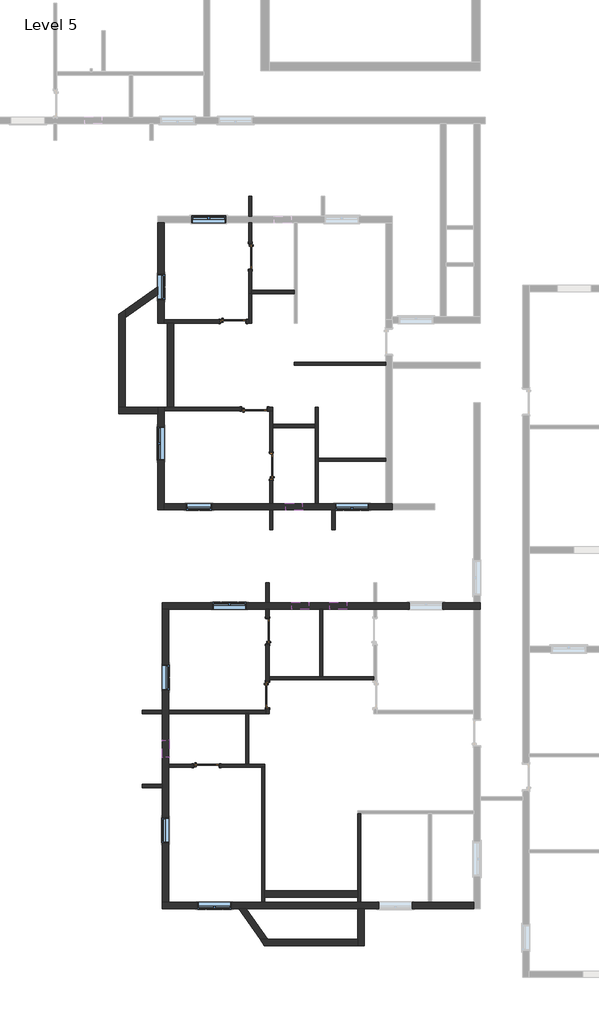
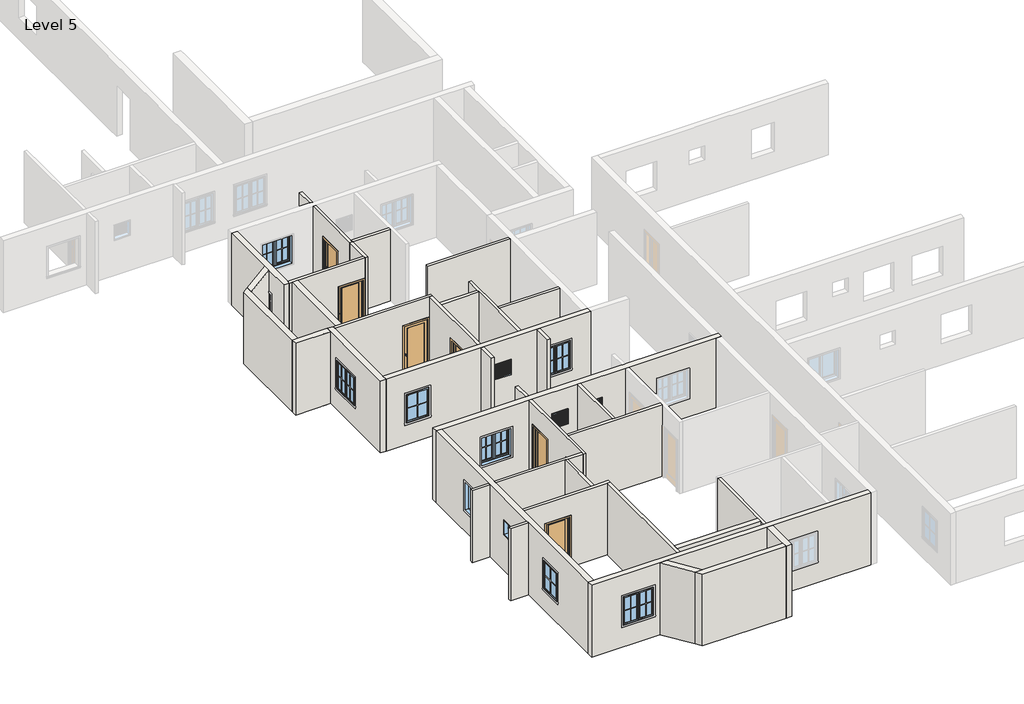
# One storey, part 1 of 7: 39 walls, 13 windows, 7 doors.
"""IFC4 building model written with IfcOpenShell, lengths in millimetres."""

from ifc_helpers import new_model, si_unit, frame, origin, place, context, project, spatial, polyline, outline, extrude, faceted_brep, transform, mapped, element, save
from components import door_3c6ab76a, door_a3feeac7, window_272f20d6, window_casement_double_4_x_4_af3140d2, window_f2d8fef0

model = new_model("IFC4")

# Units and contexts
model_context = context("Model", 3, world=origin())
ifc_project = project(units=[si_unit("LENGTHUNIT", "METRE", prefix="MILLI")], contexts=[model_context])

# Site, building, storey
site = spatial("IfcSite", under=ifc_project)
building = spatial("IfcBuilding", under=site)
storey = spatial("IfcBuildingStorey", under=building, Name="Level 5", Elevation=6400.8)

# Doors
placement = place(None, origin())
door_shape = door_3c6ab76a(model_context)
element("IfcDoor", 1, ObjectType="Door-Interior-Single-1_Panel-Wood : 2'6\" x 7' door", at=placement, inside=storey, context=model_context, shape_type="MappedRepresentation", body=[
    mapped(door_shape, transform((-4216.6759469, -3460.4538828, 6400.8), x_axis=(0.0, -1.0, 0.0), y_axis=(1.0, 0.0, 0.0), z_axis=(0.0, 0.0, 1.0))),
])
element("IfcDoor", 2, ObjectType="Door-Interior-Single-1_Panel-Wood : 2'6\" x 7' door", at=placement, inside=storey, context=model_context, shape_type="MappedRepresentation", body=[
    mapped(door_shape, transform((-5797.8259469, -21840.5288828, 6400.8), x_axis=(1.0, 0.0, 0.0), y_axis=(0.0, 1.0, 0.0), z_axis=(0.0, 0.0, 1.0))),
])
door_2_shape = door_a3feeac7(model_context)
element("IfcDoor", 3, ObjectType="Door-Interior-Single-1_Panel-Wood : 2'6\" x 7' door", at=placement, inside=storey, context=model_context, shape_type="MappedRepresentation", body=[
    mapped(door_2_shape, transform((-3454.6759469, -11032.8288828, 6400.8), x_axis=(0.0, 1.0, 0.0), y_axis=(-1.0, 0.0, 0.0), z_axis=(0.0, 0.0, 1.0))),
])
element("IfcDoor", 4, ObjectType="Door-Interior-Single-1_Panel-Wood : 2'6\" x 7' door", at=placement, inside=storey, context=model_context, shape_type="MappedRepresentation", body=[
    mapped(door_2_shape, transform((-3594.3759469, -16985.9538828, 6400.8), x_axis=(0.0, 1.0, 0.0), y_axis=(-1.0, 0.0, 0.0), z_axis=(0.0, 0.0, 1.0))),
])
element("IfcDoor", 5, ObjectType="Door-Interior-Single-1_Panel-Wood : 36\" x 84\"", at=placement, inside=storey, context=model_context, shape_type="MappedRepresentation", body=[
    mapped(door_shape, transform((-4829.4509469, -5800.4288828, 6400.8), x_axis=(1.0, 0.0, 0.0), y_axis=(0.0, 1.0, 0.0), z_axis=(0.0, 0.0, 1.0))),
])
element("IfcDoor", 6, ObjectType="Door-Interior-Single-1_Panel-Wood : 36\" x 84\"", at=placement, inside=storey, context=model_context, shape_type="MappedRepresentation", body=[
    mapped(door_2_shape, transform((-4067.4509469, -8969.0788828, 6400.8), x_axis=(1.0, 0.0, 0.0), y_axis=(0.0, 1.0, 0.0), z_axis=(0.0, 0.0, 1.0))),
])
element("IfcDoor", 7, ObjectType="Door-Interior-Single-1_Panel-Wood : 36\" x 84\"", at=placement, inside=storey, context=model_context, shape_type="MappedRepresentation", body=[
    mapped(door_2_shape, transform((-3600.7259469, -19291.0038828, 6400.8), x_axis=(0.0, -1.0, 0.0), y_axis=(1.0, 0.0, 0.0), z_axis=(0.0, 0.0, 1.0))),
])

# Walls
element("IfcWall", 8, ObjectType="4.5\" wall", at=placement, inside=storey, context=model_context, shape_type="Brep", body=[
    faceted_brep([(-4277.0009469, -4793.9538828, 9448.8), (-4277.0009469, -2241.2538828, 9448.8), (-4277.0009469, -2241.2538828, 6400.8), (-4277.0009469, -2977.8538828, 6400.8), (-4277.0009469, -2977.8538828, 8559.8), (-4277.0009469, -3943.0538828, 8559.8), (-4277.0009469, -3943.0538828, 6400.8), (-4277.0009469, -4793.9538828, 6400.8), (-4162.7009469, -2241.2538828, 9448.8), (-4162.7009469, -4679.6538828, 9448.8), (-4162.7009469, -4793.9538828, 9448.8), (-4162.7009469, -4793.9538828, 6400.8), (-4162.7009469, -4679.6538828, 6400.8), (-4162.7009469, -3943.0538828, 6400.8), (-4162.7009469, -3943.0538828, 8559.8), (-4162.7009469, -2977.8538828, 8559.8), (-4162.7009469, -2977.8538828, 6400.8), (-4162.7009469, -2241.2538828, 6400.8)], [[[0, 1, 2, 3, 4, 5, 6, 7]], [[8, 9, 10, 11, 12, 13, 14, 15, 16, 17]], [[2, 17, 16, 3]], [[11, 7, 6, 13, 12]], [[1, 0, 10, 9, 8]], [[2, 1, 8, 17]], [[0, 7, 11, 10]], [[5, 14, 13, 6]], [[14, 5, 4, 15]], [[15, 4, 3, 16]]]),
])
element("IfcWall", 9, ObjectType="4.5\" wall", at=placement, inside=storey, context=model_context, shape_type="Brep", body=[
    faceted_brep([(-4277.0009469, -4793.9538828, 6400.8), (-4277.0009469, -5746.4538828, 6400.8), (-4277.0009469, -5860.7538828, 6400.8), (-4277.0009469, -5860.7538828, 9448.8), (-4277.0009469, -5746.4538828, 9448.8), (-4277.0009469, -4793.9538828, 9448.8), (-4162.7009469, -4793.9538828, 6400.8), (-4162.7009469, -4793.9538828, 9448.8), (-4162.7009469, -5860.7538828, 9448.8), (-4162.7009469, -5860.7538828, 6400.8)], [[[0, 1, 2, 3, 4, 5]], [[6, 7, 8, 9]], [[2, 1, 0, 6, 9]], [[5, 4, 3, 8, 7]], [[0, 5, 7, 6]], [[3, 2, 9, 8]]]),
])
element("IfcWall", 10, ObjectType="4.5\" wall", at=placement, inside=storey, context=model_context, shape_type="Brep", body=[
    faceted_brep([(-7325.0009469, -5746.4538828, 9448.8), (-4277.0009469, -5746.4538828, 9448.8), (-4277.0009469, -5746.4538828, 6400.8), (-4346.8509469, -5746.4538828, 6400.8), (-4346.8509469, -5746.4538828, 8559.8), (-5312.0509469, -5746.4538828, 8559.8), (-5312.0509469, -5746.4538828, 6400.8), (-7325.0009469, -5746.4538828, 6400.8), (-4277.0009469, -5860.7538828, 9448.8), (-6982.1009469, -5860.7538828, 9448.8), (-7210.7009469, -5860.7538828, 9448.8), (-7325.0009469, -5860.7538828, 9448.8), (-7325.0009469, -5860.7538828, 6400.8), (-7210.7009469, -5860.7538828, 6400.8), (-6982.1009469, -5860.7538828, 6400.8), (-5312.0509469, -5860.7538828, 6400.8), (-5312.0509469, -5860.7538828, 8559.8), (-4346.8509469, -5860.7538828, 8559.8), (-4346.8509469, -5860.7538828, 6400.8), (-4277.0009469, -5860.7538828, 6400.8)], [[[0, 1, 2, 3, 4, 5, 6, 7]], [[8, 9, 10, 11, 12, 13, 14, 15, 16, 17, 18, 19]], [[12, 7, 6, 15, 14, 13]], [[2, 19, 18, 3]], [[1, 0, 11, 10, 9, 8]], [[0, 7, 12, 11]], [[2, 1, 8, 19]], [[17, 4, 3, 18]], [[4, 17, 16, 5]], [[5, 16, 15, 6]]]),
])
element("IfcWall", 11, ObjectType="4.5\" wall", at=placement, inside=storey, context=model_context, shape_type="SweptSolid", body=[
    extrude(outline(polyline([(-2638.7009469, -4793.9538828), (-4162.7009469, -4793.9538828), (-4162.7009469, -4679.6538828), (-2638.7009469, -4679.6538828), (-2638.7009469, -4793.9538828)])), frame((0.0, 0.0, 6400.8), z_axis=(0.0, 0.0, 1.0), x_axis=(1.0, 0.0, 0.0)), (0.0, 0.0, 1.0), 3048.0),
])
element("IfcWall", 12, ObjectType="4.5\" wall", at=placement, inside=storey, context=model_context, shape_type="SweptSolid", body=[
    extrude(outline(polyline([(-2638.7009469, -7270.4538828), (675.9990531, -7270.4538828), (675.9990531, -7384.7538828), (-2638.7009469, -7384.7538828), (-2638.7009469, -7270.4538828)])), frame((0.0, 0.0, 6400.8), z_axis=(0.0, 0.0, 1.0), x_axis=(1.0, 0.0, 0.0)), (0.0, 0.0, 1.0), 3048.0),
])
element("IfcWall", 13, ObjectType="4.5\" wall", at=placement, inside=storey, context=model_context, shape_type="Brep", body=[
    faceted_brep([(-7325.0009469, -8908.7538828, 9448.8), (-7210.7009469, -8908.7538828, 9448.8), (-6982.1009469, -8908.7538828, 9448.8), (-3400.7009469, -8908.7538828, 9448.8), (-3400.7009469, -8908.7538828, 6400.8), (-3584.8509469, -8908.7538828, 6400.8), (-3584.8509469, -8908.7538828, 8559.8), (-4550.0509469, -8908.7538828, 8559.8), (-4550.0509469, -8908.7538828, 6400.8), (-6982.1009469, -8908.7538828, 6400.8), (-7210.7009469, -8908.7538828, 6400.8), (-7325.0009469, -8908.7538828, 6400.8), (-3400.7009469, -9023.0538828, 9448.8), (-3515.0009469, -9023.0538828, 9448.8), (-7325.0009469, -9023.0538828, 9448.8), (-7325.0009469, -9023.0538828, 6400.8), (-4550.0509469, -9023.0538828, 6400.8), (-4550.0509469, -9023.0538828, 8559.8), (-3584.8509469, -9023.0538828, 8559.8), (-3584.8509469, -9023.0538828, 6400.8), (-3515.0009469, -9023.0538828, 6400.8), (-3400.7009469, -9023.0538828, 6400.8)], [[[0, 1, 2, 3, 4, 5, 6, 7, 8, 9, 10, 11]], [[12, 13, 14, 15, 16, 17, 18, 19, 20, 21]], [[4, 21, 20, 19, 5]], [[15, 11, 10, 9, 8, 16]], [[3, 2, 1, 0, 14, 13, 12]], [[4, 3, 12, 21]], [[0, 11, 15, 14]], [[18, 6, 5, 19]], [[6, 18, 17, 7]], [[7, 17, 16, 8]]]),
])
element("IfcWall", 14, ObjectType="4.5\" wall", at=placement, inside=storey, context=model_context, shape_type="SweptSolid", body=[
    extrude(outline(polyline([(-1876.7009469, -9632.6538828), (-3400.7009469, -9632.6538828), (-3400.7009469, -9518.3538828), (-1876.7009469, -9518.3538828), (-1876.7009469, -9632.6538828)])), frame((0.0, 0.0, 6400.8), z_axis=(0.0, 0.0, 1.0), x_axis=(1.0, 0.0, 0.0)), (0.0, 0.0, 1.0), 3048.0),
])
element("IfcWall", 15, ObjectType="4.5\" wall", at=placement, inside=storey, context=model_context, shape_type="Brep", body=[
    faceted_brep([(-1762.4009469, -12375.8538828, 6400.8), (-1762.4009469, -10851.8538828, 6400.8), (-1762.4009469, -10737.5538828, 6400.8), (-1762.4009469, -8908.7538828, 6400.8), (-1762.4009469, -8908.7538828, 9448.8), (-1762.4009469, -10737.5538828, 9448.8), (-1762.4009469, -10851.8538828, 9448.8), (-1762.4009469, -12375.8538828, 9448.8), (-1876.7009469, -12375.8538828, 6400.8), (-1876.7009469, -12375.8538828, 9448.8), (-1876.7009469, -9632.6538828, 9448.8), (-1876.7009469, -9518.3538828, 9448.8), (-1876.7009469, -8908.7538828, 9448.8), (-1876.7009469, -8908.7538828, 6400.8), (-1876.7009469, -9518.3538828, 6400.8), (-1876.7009469, -9632.6538828, 6400.8)], [[[0, 1, 2, 3, 4, 5, 6, 7]], [[8, 9, 10, 11, 12, 13, 14, 15]], [[3, 2, 1, 0, 8, 15, 14, 13]], [[4, 3, 13, 12]], [[7, 6, 5, 4, 12, 11, 10, 9]], [[0, 7, 9, 8]]]),
])
element("IfcWall", 16, ObjectType="4.5\" wall", at=placement, inside=storey, context=model_context, shape_type="Brep", body=[
    faceted_brep([(-3400.7009469, -9023.0538828, 9448.8), (-3400.7009469, -9518.3538828, 9448.8), (-3400.7009469, -9632.6538828, 9448.8), (-3400.7009469, -12375.8538828, 9448.8), (-3400.7009469, -12375.8538828, 6400.8), (-3400.7009469, -11515.4288828, 6400.8), (-3400.7009469, -11515.4288828, 8559.8), (-3400.7009469, -10550.2288828, 8559.8), (-3400.7009469, -10550.2288828, 6400.8), (-3400.7009469, -9632.6538828, 6400.8), (-3400.7009469, -9518.3538828, 6400.8), (-3400.7009469, -9023.0538828, 6400.8), (-3515.0009469, -12375.8538828, 9448.8), (-3515.0009469, -9023.0538828, 9448.8), (-3515.0009469, -9023.0538828, 6400.8), (-3515.0009469, -10550.2288828, 6400.8), (-3515.0009469, -10550.2288828, 8559.8), (-3515.0009469, -11515.4288828, 8559.8), (-3515.0009469, -11515.4288828, 6400.8), (-3515.0009469, -12375.8538828, 6400.8)], [[[0, 1, 2, 3, 4, 5, 6, 7, 8, 9, 10, 11]], [[12, 13, 14, 15, 16, 17, 18, 19]], [[4, 19, 18, 5]], [[14, 11, 10, 9, 8, 15]], [[3, 2, 1, 0, 13, 12]], [[4, 3, 12, 19]], [[0, 11, 14, 13]], [[7, 16, 15, 8]], [[16, 7, 6, 17]], [[17, 6, 5, 18]]]),
])
element("IfcWall", 17, ObjectType="4.5\" wall", at=placement, inside=storey, context=model_context, shape_type="SweptSolid", body=[
    extrude(outline(polyline([(-1762.4009469, -10737.5538828), (675.9990531, -10737.5538828), (675.9990531, -10851.8538828), (-1762.4009469, -10851.8538828), (-1762.4009469, -10737.5538828)])), frame((0.0, 0.0, 6400.8), z_axis=(0.0, 0.0, 1.0), x_axis=(1.0, 0.0, 0.0)), (0.0, 0.0, 1.0), 3048.0),
])
element("IfcWall", 18, ObjectType="4.5\" wall", at=placement, inside=storey, context=model_context, shape_type="SweptSolid", body=[
    extrude(outline(polyline([(-3515.0009469, -13328.3538828), (-3515.0009469, -12604.4538828), (-3400.7009469, -12604.4538828), (-3400.7009469, -13328.3538828), (-3515.0009469, -13328.3538828)])), frame((0.0, 0.0, 6400.8), z_axis=(0.0, 0.0, 1.0), x_axis=(1.0, 0.0, 0.0)), (0.0, 0.0, 1.0), 3048.0),
])
element("IfcWall", 19, ObjectType="4.5\" wall", at=placement, inside=storey, context=model_context, shape_type="Brep", body=[
    faceted_brep([(-1152.8009469, -13328.3538828, 6400.8), (-1152.8009469, -12604.4538828, 6400.8), (-1152.8009469, -12604.4538828, 7315.2), (-1152.8009469, -12604.4538828, 8534.4), (-1152.8009469, -12604.4538828, 9448.8), (-1152.8009469, -13328.3538828, 9448.8), (-1267.1009469, -13328.3538828, 6400.8), (-1267.1009469, -13328.3538828, 9448.8), (-1267.1009469, -12604.4538828, 9448.8), (-1267.1009469, -12604.4538828, 6400.8)], [[[0, 1, 2, 3, 4, 5]], [[6, 7, 8, 9]], [[1, 0, 6, 9]], [[5, 4, 8, 7]], [[0, 5, 7, 6]], [[4, 3, 2, 1, 9, 8]]]),
])
element("IfcWall", 20, ObjectType="4.5\" wall", at=placement, inside=storey, context=model_context, shape_type="SweptSolid", body=[
    extrude(outline(polyline([(-4162.7009469, -1288.7538828), (-4162.7009469, -2012.6538828), (-4277.0009469, -2012.6538828), (-4277.0009469, -1288.7538828), (-4162.7009469, -1288.7538828)])), frame((0.0, 0.0, 6400.8), z_axis=(0.0, 0.0, 1.0), x_axis=(1.0, 0.0, 0.0)), (0.0, 0.0, 1.0), 3048.0),
])
element("IfcWall", 21, ObjectType="4.5\" wall", at=placement, inside=storey, context=model_context, shape_type="Brep", body=[
    faceted_brep([(231.4990531, -18624.2538828, 6400.8), (-1597.3009469, -18624.2538828, 6400.8), (-1711.6009469, -18624.2538828, 6400.8), (-3540.4009469, -18624.2538828, 6400.8), (-3540.4009469, -18624.2538828, 9448.8), (-1711.6009469, -18624.2538828, 9448.8), (-1597.3009469, -18624.2538828, 9448.8), (231.4990531, -18624.2538828, 9448.8), (231.4990531, -18738.5538828, 6400.8), (231.4990531, -18738.5538828, 9448.8), (-3540.4009469, -18738.5538828, 9448.8), (-3540.4009469, -18738.5538828, 6400.8)], [[[0, 1, 2, 3, 4, 5, 6, 7]], [[8, 9, 10, 11]], [[3, 2, 1, 0, 8, 11]], [[7, 6, 5, 4, 10, 9]], [[4, 3, 11, 10]], [[0, 7, 9, 8]]]),
])
element("IfcWall", 22, ObjectType="4.5\" wall", at=placement, inside=storey, context=model_context, shape_type="SweptSolid", body=[
    extrude(outline(polyline([(-1597.3009469, -16185.8538828), (-1597.3009469, -18624.2538828), (-1711.6009469, -18624.2538828), (-1711.6009469, -16185.8538828), (-1597.3009469, -16185.8538828)])), frame((0.0, 0.0, 6400.8), z_axis=(0.0, 0.0, 1.0), x_axis=(1.0, 0.0, 0.0)), (0.0, 0.0, 1.0), 3048.0),
])
element("IfcWall", 23, ObjectType="4.5\" wall", at=placement, inside=storey, context=model_context, shape_type="SweptSolid", body=[
    extrude(outline(polyline([(-3540.4009469, -15233.3538828), (-3540.4009469, -15957.2538828), (-3654.7009469, -15957.2538828), (-3654.7009469, -15233.3538828), (-3540.4009469, -15233.3538828)])), frame((0.0, 0.0, 6400.8), z_axis=(0.0, 0.0, 1.0), x_axis=(1.0, 0.0, 0.0)), (0.0, 0.0, 1.0), 3048.0),
])
element("IfcWall", 24, ObjectType="4.5\" wall", at=placement, inside=storey, context=model_context, shape_type="Brep", body=[
    faceted_brep([(-3654.7009469, -19957.7538828, 9448.8), (-3654.7009469, -19843.4538828, 9448.8), (-3654.7009469, -16185.8538828, 9448.8), (-3654.7009469, -16185.8538828, 6400.8), (-3654.7009469, -16503.3538828, 6400.8), (-3654.7009469, -16503.3538828, 8559.8), (-3654.7009469, -17468.5538828, 8559.8), (-3654.7009469, -17468.5538828, 6400.8), (-3654.7009469, -18808.4038828, 6400.8), (-3654.7009469, -18808.4038828, 8559.8), (-3654.7009469, -19773.6038828, 8559.8), (-3654.7009469, -19773.6038828, 6400.8), (-3654.7009469, -19843.4538828, 6400.8), (-3654.7009469, -19957.7538828, 6400.8), (-3540.4009469, -16185.8538828, 9448.8), (-3540.4009469, -18624.2538828, 9448.8), (-3540.4009469, -18738.5538828, 9448.8), (-3540.4009469, -19957.7538828, 9448.8), (-3540.4009469, -19957.7538828, 6400.8), (-3540.4009469, -19773.6038828, 6400.8), (-3540.4009469, -19773.6038828, 8559.8), (-3540.4009469, -18808.4038828, 8559.8), (-3540.4009469, -18808.4038828, 6400.8), (-3540.4009469, -18738.5538828, 6400.8), (-3540.4009469, -18624.2538828, 6400.8), (-3540.4009469, -17468.5538828, 6400.8), (-3540.4009469, -17468.5538828, 8559.8), (-3540.4009469, -16503.3538828, 8559.8), (-3540.4009469, -16503.3538828, 6400.8), (-3540.4009469, -16185.8538828, 6400.8)], [[[0, 1, 2, 3, 4, 5, 6, 7, 8, 9, 10, 11, 12, 13]], [[14, 15, 16, 17, 18, 19, 20, 21, 22, 23, 24, 25, 26, 27, 28, 29]], [[3, 29, 28, 4]], [[18, 13, 12, 11, 19]], [[7, 25, 24, 23, 22, 8]], [[2, 1, 0, 17, 16, 15, 14]], [[3, 2, 14, 29]], [[0, 13, 18, 17]], [[27, 5, 4, 28]], [[5, 27, 26, 6]], [[6, 26, 25, 7]], [[10, 20, 19, 11]], [[20, 10, 9, 21]], [[21, 9, 8, 22]]]),
])
element("IfcWall", 25, ObjectType="4.5\" wall", at=placement, inside=storey, context=model_context, shape_type="Brep", body=[
    faceted_brep([(-3654.7009469, -19843.4538828, 6400.8), (-7159.9009469, -19843.4538828, 6400.8), (-7159.9009469, -19843.4538828, 9448.8), (-3654.7009469, -19843.4538828, 9448.8), (-3654.7009469, -19957.7538828, 6400.8), (-3654.7009469, -19957.7538828, 9448.8), (-4264.3009469, -19957.7538828, 9448.8), (-4378.6009469, -19957.7538828, 9448.8), (-7159.9009469, -19957.7538828, 9448.8), (-7159.9009469, -19957.7538828, 6400.8), (-4378.6009469, -19957.7538828, 6400.8), (-4264.3009469, -19957.7538828, 6400.8)], [[[0, 1, 2, 3]], [[4, 5, 6, 7, 8, 9, 10, 11]], [[1, 0, 4, 11, 10, 9]], [[3, 2, 8, 7, 6, 5]], [[2, 1, 9, 8]], [[0, 3, 5, 4]]]),
])
element("IfcWall", 26, ObjectType="4.5\" wall", at=placement, inside=storey, context=model_context, shape_type="Brep", body=[
    faceted_brep([(-7159.9009469, -21786.5538828, 9448.8), (-4378.6009469, -21786.5538828, 9448.8), (-4264.3009469, -21786.5538828, 9448.8), (-3692.8009469, -21786.5538828, 9448.8), (-3692.8009469, -21786.5538828, 6400.8), (-4264.3009469, -21786.5538828, 6400.8), (-4378.6009469, -21786.5538828, 6400.8), (-5315.2259469, -21786.5538828, 6400.8), (-5315.2259469, -21786.5538828, 8559.8), (-6280.4259469, -21786.5538828, 8559.8), (-6280.4259469, -21786.5538828, 6400.8), (-7159.9009469, -21786.5538828, 6400.8), (-3692.8009469, -21900.8538828, 9448.8), (-3807.1009469, -21900.8538828, 9448.8), (-7159.9009469, -21900.8538828, 9448.8), (-7159.9009469, -21900.8538828, 6400.8), (-6280.4259469, -21900.8538828, 6400.8), (-6280.4259469, -21900.8538828, 8559.8), (-5315.2259469, -21900.8538828, 8559.8), (-5315.2259469, -21900.8538828, 6400.8), (-3807.1009469, -21900.8538828, 6400.8), (-3692.8009469, -21900.8538828, 6400.8)], [[[0, 1, 2, 3, 4, 5, 6, 7, 8, 9, 10, 11]], [[12, 13, 14, 15, 16, 17, 18, 19, 20, 21]], [[15, 11, 10, 16]], [[4, 21, 20, 19, 7, 6, 5]], [[3, 2, 1, 0, 14, 13, 12]], [[0, 11, 15, 14]], [[4, 3, 12, 21]], [[18, 8, 7, 19]], [[8, 18, 17, 9]], [[9, 17, 16, 10]]]),
])
element("IfcWall", 27, ObjectType="4.5\" wall", at=placement, inside=storey, context=model_context, shape_type="Brep", body=[
    faceted_brep([(-3692.8009469, -26777.6538828, 6400.8), (-3692.8009469, -26587.1538828, 6400.8), (-3692.8009469, -26358.5538828, 6400.8), (-3692.8009469, -21900.8538828, 6400.8), (-3692.8009469, -21900.8538828, 9448.8), (-3692.8009469, -26358.5538828, 9448.8), (-3692.8009469, -26587.1538828, 9448.8), (-3692.8009469, -26777.6538828, 9448.8), (-3807.1009469, -26777.6538828, 6400.8), (-3807.1009469, -26777.6538828, 9448.8), (-3807.1009469, -21900.8538828, 9448.8), (-3807.1009469, -21900.8538828, 6400.8)], [[[0, 1, 2, 3, 4, 5, 6, 7]], [[8, 9, 10, 11]], [[3, 2, 1, 0, 8, 11]], [[7, 6, 5, 4, 10, 9]], [[4, 3, 11, 10]], [[0, 7, 9, 8]]]),
])
element("IfcWall", 28, ObjectType="4.5\" wall", at=placement, inside=storey, context=model_context, shape_type="SweptSolid", body=[
    extrude(outline(polyline([(-7388.5009469, -22629.8863256), (-8112.4009469, -22629.8863256), (-8112.4009469, -22515.5863256), (-7388.5009469, -22515.5863256), (-7388.5009469, -22629.8863256)])), frame((0.0, 0.0, 6400.8), z_axis=(0.0, 0.0, 1.0), x_axis=(1.0, 0.0, 0.0)), (0.0, 0.0, 1.0), 3048.0),
])
element("IfcWall", 29, ObjectType="4.5\" wall", at=placement, inside=storey, context=model_context, shape_type="SweptSolid", body=[
    extrude(outline(polyline([(-8112.4009469, -19843.4538828), (-7388.5009469, -19843.4538828), (-7388.5009469, -19957.7538828), (-8112.4009469, -19957.7538828), (-8112.4009469, -19843.4538828)])), frame((0.0, 0.0, 6400.8), z_axis=(0.0, 0.0, 1.0), x_axis=(1.0, 0.0, 0.0)), (0.0, 0.0, 1.0), 3048.0),
])
element("IfcWall", 30, ObjectType="4.5\" wall", at=placement, inside=storey, context=model_context, shape_type="SweptSolid", body=[
    extrude(outline(polyline([(-4378.6009469, -21786.5538828), (-4378.6009469, -19957.7538828), (-4264.3009469, -19957.7538828), (-4264.3009469, -21786.5538828), (-4378.6009469, -21786.5538828)])), frame((0.0, 0.0, 6400.8), z_axis=(0.0, 0.0, 1.0), x_axis=(1.0, 0.0, 0.0)), (0.0, 0.0, 1.0), 3048.0),
])
element("IfcWall", 31, ObjectType="4.5\" wall", at=placement, inside=storey, context=model_context, shape_type="Brep", body=[
    faceted_brep([(-340.0009469, -23577.2538828, 6400.8), (-340.0009469, -26358.5538828, 6400.8), (-340.0009469, -26587.1538828, 6400.8), (-340.0009469, -26777.6538828, 6400.8), (-340.0009469, -26777.6538828, 9448.8), (-340.0009469, -26587.1538828, 9448.8), (-340.0009469, -26358.5538828, 9448.8), (-340.0009469, -23577.2538828, 9448.8), (-225.7009469, -23577.2538828, 6400.8), (-225.7009469, -23577.2538828, 9448.8), (-225.7009469, -26777.6538828, 9448.8), (-225.7009469, -26777.6538828, 6400.8)], [[[0, 1, 2, 3, 4, 5, 6, 7]], [[8, 9, 10, 11]], [[3, 2, 1, 0, 8, 11]], [[7, 6, 5, 4, 10, 9]], [[0, 7, 9, 8]], [[4, 3, 11, 10]]]),
])
element("IfcWall", 32, ObjectType="9\"", at=placement, inside=storey, context=model_context, shape_type="Brep", body=[
    faceted_brep([(-7553.6009469, -2241.2538828, 6400.8), (-7553.6009469, -4556.8220214, 6400.8), (-7553.6009469, -4835.8638828, 6400.8), (-7553.6009469, -5860.7538828, 6400.8), (-7553.6009469, -5860.7538828, 9448.8), (-7553.6009469, -4835.8638828, 9448.8), (-7553.6009469, -4556.8220214, 9448.8), (-7553.6009469, -2241.2538828, 9448.8), (-7553.6009469, -5016.2038828, 8534.4), (-7553.6009469, -5016.2038828, 7315.2), (-7553.6009469, -4101.8038828, 7315.2), (-7553.6009469, -4101.8038828, 8534.4), (-7325.0009469, -2241.2538828, 6400.8), (-7325.0009469, -2241.2538828, 9448.8), (-7325.0009469, -5746.4538828, 9448.8), (-7325.0009469, -5860.7538828, 9448.8), (-7325.0009469, -5860.7538828, 6400.8), (-7325.0009469, -5746.4538828, 6400.8), (-7325.0009469, -5016.2038828, 8534.4), (-7325.0009469, -4101.8038828, 8534.4), (-7325.0009469, -4101.8038828, 7315.2), (-7325.0009469, -5016.2038828, 7315.2)], [[[0, 1, 2, 3, 4, 5, 6, 7], [8, 9, 10, 11]], [[12, 13, 14, 15, 16, 17], [18, 19, 20, 21]], [[3, 2, 1, 0, 12, 17, 16]], [[7, 6, 5, 4, 15, 14, 13]], [[0, 7, 13, 12]], [[4, 3, 16, 15]], [[9, 8, 18, 21]], [[10, 9, 21, 20]], [[11, 10, 20, 19]], [[8, 11, 19, 18]]]),
])
element("IfcWall", 33, ObjectType="9\"", at=placement, inside=storey, context=model_context, shape_type="SweptSolid", body=[
    extrude(outline(polyline([(-6982.1009469, -5860.7538828), (-6982.1009469, -8908.7538828), (-7210.7009469, -8908.7538828), (-7210.7009469, -5860.7538828), (-6982.1009469, -5860.7538828)])), frame((0.0, 0.0, 6400.8), z_axis=(0.0, 0.0, 1.0), x_axis=(1.0, 0.0, 0.0)), (0.0, 0.0, 1.0), 3048.0),
])
element("IfcWall", 34, ObjectType="9\"", at=placement, inside=storey, context=model_context, shape_type="Brep", body=[
    faceted_brep([(-7553.6009469, -8908.7538828, 6400.8), (-7553.6009469, -9137.3538828, 6400.8), (-7553.6009469, -12604.4538828, 6400.8), (-7553.6009469, -12604.4538828, 9448.8), (-7553.6009469, -9137.3538828, 9448.8), (-7553.6009469, -8908.7538828, 9448.8), (-7553.6009469, -9600.9038828, 8534.4), (-7553.6009469, -10820.1038828, 8534.4), (-7553.6009469, -10820.1038828, 7315.2), (-7553.6009469, -9600.9038828, 7315.2), (-7325.0009469, -8908.7538828, 6400.8), (-7325.0009469, -8908.7538828, 9448.8), (-7325.0009469, -9023.0538828, 9448.8), (-7325.0009469, -12375.8538828, 9448.8), (-7325.0009469, -12604.4538828, 9448.8), (-7325.0009469, -12604.4538828, 6400.8), (-7325.0009469, -12375.8538828, 6400.8), (-7325.0009469, -9023.0538828, 6400.8), (-7325.0009469, -9600.9038828, 8534.4), (-7325.0009469, -9600.9038828, 7315.2), (-7325.0009469, -10820.1038828, 7315.2), (-7325.0009469, -10820.1038828, 8534.4)], [[[0, 1, 2, 3, 4, 5], [6, 7, 8, 9]], [[10, 11, 12, 13, 14, 15, 16, 17], [18, 19, 20, 21]], [[2, 1, 0, 10, 17, 16, 15]], [[5, 4, 3, 14, 13, 12, 11]], [[3, 2, 15, 14]], [[0, 5, 11, 10]], [[19, 18, 6, 9]], [[20, 19, 9, 8]], [[21, 20, 8, 7]], [[18, 21, 7, 6]]]),
])
element("IfcWall", 35, ObjectType="9\"", at=placement, inside=storey, context=model_context, shape_type="Brep", body=[
    faceted_brep([(-7325.0009469, -12604.4538828, 6400.8), (-3515.0009469, -12604.4538828, 6400.8), (-3400.7009469, -12604.4538828, 6400.8), (-1267.1009469, -12604.4538828, 6400.8), (-1152.8009469, -12604.4538828, 6400.8), (904.5990531, -12604.4538828, 6400.8), (904.5990531, -12604.4538828, 9448.8), (-1152.8009469, -12604.4538828, 9448.8), (-1267.1009469, -12604.4538828, 9448.8), (-3400.7009469, -12604.4538828, 9448.8), (-3515.0009469, -12604.4538828, 9448.8), (-7325.0009469, -12604.4538828, 9448.8), (-2333.9009469, -12604.4538828, 8534.4), (-2333.9009469, -12604.4538828, 7924.8), (-2943.5009469, -12604.4538828, 7924.8), (-2943.5009469, -12604.4538828, 8534.4), (-6524.9009469, -12604.4538828, 8534.4), (-5610.5009469, -12604.4538828, 8534.4), (-5610.5009469, -12604.4538828, 7315.2), (-6524.9009469, -12604.4538828, 7315.2), (-1152.8009469, -12604.4538828, 8534.4), (66.3990531, -12604.4538828, 8534.4), (66.3990531, -12604.4538828, 7315.2), (-1152.8009469, -12604.4538828, 7315.2), (-7325.0009469, -12375.8538828, 6400.8), (-7325.0009469, -12375.8538828, 9448.8), (-3515.0009469, -12375.8538828, 9448.8), (-3400.7009469, -12375.8538828, 9448.8), (-1876.7009469, -12375.8538828, 9448.8), (-1762.4009469, -12375.8538828, 9448.8), (675.9990531, -12375.8538828, 9448.8), (904.5990531, -12375.8538828, 9448.8), (904.5990531, -12375.8538828, 6400.8), (675.9990531, -12375.8538828, 6400.8), (-1762.4009469, -12375.8538828, 6400.8), (-1876.7009469, -12375.8538828, 6400.8), (-3400.7009469, -12375.8538828, 6400.8), (-3515.0009469, -12375.8538828, 6400.8), (-2333.9009469, -12375.8538828, 8534.4), (-2943.5009469, -12375.8538828, 8534.4), (-2943.5009469, -12375.8538828, 7924.8), (-2333.9009469, -12375.8538828, 7924.8), (-6524.9009469, -12375.8538828, 8534.4), (-6524.9009469, -12375.8538828, 7315.2), (-5610.5009469, -12375.8538828, 7315.2), (-5610.5009469, -12375.8538828, 8534.4), (-1152.8009469, -12375.8538828, 8534.4), (-1152.8009469, -12375.8538828, 7315.2), (66.3990531, -12375.8538828, 7315.2), (66.3990531, -12375.8538828, 8534.4)], [[[0, 1, 2, 3, 4, 5, 6, 7, 8, 9, 10, 11], [12, 13, 14, 15], [16, 17, 18, 19], [20, 21, 22, 23]], [[24, 25, 26, 27, 28, 29, 30, 31, 32, 33, 34, 35, 36, 37], [38, 39, 40, 41], [42, 43, 44, 45], [46, 47, 48, 49]], [[5, 4, 3, 2, 1, 0, 24, 37, 36, 35, 34, 33, 32]], [[11, 10, 9, 8, 7, 6, 31, 30, 29, 28, 27, 26, 25]], [[0, 11, 25, 24]], [[6, 5, 32, 31]], [[13, 12, 38, 41]], [[14, 13, 41, 40]], [[15, 14, 40, 39]], [[12, 15, 39, 38]], [[43, 42, 16, 19]], [[44, 43, 19, 18]], [[45, 44, 18, 17]], [[42, 45, 17, 16]], [[47, 46, 20, 23]], [[48, 47, 23, 22]], [[49, 48, 22, 21]], [[46, 49, 21, 20]]]),
])
element("IfcWall", 36, ObjectType="9\"", at=placement, inside=storey, context=model_context, shape_type="SweptSolid", body=[
    extrude(outline(polyline([(-7820.3009469, -8908.7538828), (-7553.6009469, -8908.7538828), (-7553.6009469, -9137.3538828), (-7820.3009469, -9137.3538828), (-7820.3009469, -8908.7538828)])), frame((0.0, 0.0, 6400.8), z_axis=(0.0, 0.0, 1.0), x_axis=(1.0, 0.0, 0.0)), (0.0, 0.0, 1.0), 3048.0),
])
element("IfcWall", 37, ObjectType="9\"", at=placement, inside=storey, context=model_context, shape_type="Brep", body=[
    faceted_brep([(-7388.5009469, -16185.8538828, 6400.8), (-7159.9009469, -16185.8538828, 6400.8), (-3654.7009469, -16185.8538828, 6400.8), (-3540.4009469, -16185.8538828, 6400.8), (-1711.6009469, -16185.8538828, 6400.8), (-1597.3009469, -16185.8538828, 6400.8), (231.4990531, -16185.8538828, 6400.8), (345.7990531, -16185.8538828, 6400.8), (3850.9990531, -16185.8538828, 6400.8), (4079.5990531, -16185.8538828, 6400.8), (4079.5990531, -16185.8538828, 9448.8), (3850.9990531, -16185.8538828, 9448.8), (345.7990531, -16185.8538828, 9448.8), (231.4990531, -16185.8538828, 9448.8), (-1597.3009469, -16185.8538828, 9448.8), (-1711.6009469, -16185.8538828, 9448.8), (-3540.4009469, -16185.8538828, 9448.8), (-3654.7009469, -16185.8538828, 9448.8), (-7159.9009469, -16185.8538828, 9448.8), (-7388.5009469, -16185.8538828, 9448.8), (-740.0509469, -16185.8538828, 8534.4), (-740.0509469, -16185.8538828, 7924.8), (-1349.6509469, -16185.8538828, 7924.8), (-1349.6509469, -16185.8538828, 8534.4), (-2111.6509469, -16185.8538828, 8534.4), (-2111.6509469, -16185.8538828, 7924.8), (-2721.2509469, -16185.8538828, 7924.8), (-2721.2509469, -16185.8538828, 8534.4), (2736.5740531, -16185.8538828, 8534.4), (2736.5740531, -16185.8538828, 7315.2), (1517.3740531, -16185.8538828, 7315.2), (1517.3740531, -16185.8538828, 8534.4), (-4359.5509469, -16185.8538828, 8534.4), (-4359.5509469, -16185.8538828, 7315.2), (-5578.7509469, -16185.8538828, 7315.2), (-5578.7509469, -16185.8538828, 8534.4), (-7388.5009469, -15957.2538828, 6400.8), (-7388.5009469, -15957.2538828, 9448.8), (-3654.7009469, -15957.2538828, 9448.8), (-3540.4009469, -15957.2538828, 9448.8), (231.4990531, -15957.2538828, 9448.8), (345.7990531, -15957.2538828, 9448.8), (3850.9990531, -15957.2538828, 9448.8), (4079.5990531, -15957.2538828, 9448.8), (4079.5990531, -15957.2538828, 6400.8), (3850.9990531, -15957.2538828, 6400.8), (345.7990531, -15957.2538828, 6400.8), (231.4990531, -15957.2538828, 6400.8), (-3540.4009469, -15957.2538828, 6400.8), (-3654.7009469, -15957.2538828, 6400.8), (-740.0509469, -15957.2538828, 8534.4), (-1349.6509469, -15957.2538828, 8534.4), (-1349.6509469, -15957.2538828, 7924.8), (-740.0509469, -15957.2538828, 7924.8), (-2111.6509469, -15957.2538828, 8534.4), (-2721.2509469, -15957.2538828, 8534.4), (-2721.2509469, -15957.2538828, 7924.8), (-2111.6509469, -15957.2538828, 7924.8), (2736.5740531, -15957.2538828, 8534.4), (1517.3740531, -15957.2538828, 8534.4), (1517.3740531, -15957.2538828, 7315.2), (2736.5740531, -15957.2538828, 7315.2), (-4359.5509469, -15957.2538828, 8534.4), (-5578.7509469, -15957.2538828, 8534.4), (-5578.7509469, -15957.2538828, 7315.2), (-4359.5509469, -15957.2538828, 7315.2)], [[[0, 1, 2, 3, 4, 5, 6, 7, 8, 9, 10, 11, 12, 13, 14, 15, 16, 17, 18, 19], [20, 21, 22, 23], [24, 25, 26, 27], [28, 29, 30, 31], [32, 33, 34, 35]], [[36, 37, 38, 39, 40, 41, 42, 43, 44, 45, 46, 47, 48, 49], [50, 51, 52, 53], [54, 55, 56, 57], [58, 59, 60, 61], [62, 63, 64, 65]], [[9, 8, 7, 6, 5, 4, 3, 2, 1, 0, 36, 49, 48, 47, 46, 45, 44]], [[19, 18, 17, 16, 15, 14, 13, 12, 11, 10, 43, 42, 41, 40, 39, 38, 37]], [[0, 19, 37, 36]], [[10, 9, 44, 43]], [[21, 20, 50, 53]], [[22, 21, 53, 52]], [[23, 22, 52, 51]], [[20, 23, 51, 50]], [[25, 24, 54, 57]], [[26, 25, 57, 56]], [[27, 26, 56, 55]], [[24, 27, 55, 54]], [[29, 28, 58, 61]], [[30, 29, 61, 60]], [[31, 30, 60, 59]], [[28, 31, 59, 58]], [[33, 32, 62, 65]], [[34, 33, 65, 64]], [[35, 34, 64, 63]], [[32, 35, 63, 62]]]),
])
element("IfcWall", 38, ObjectType="9\"", at=placement, inside=storey, context=model_context, shape_type="Brep", body=[
    faceted_brep([(3850.9990531, -26777.6538828, 6400.8), (2326.9990531, -26777.6538828, 6400.8), (2212.6990531, -26777.6538828, 6400.8), (-225.7009469, -26777.6538828, 6400.8), (-340.0009469, -26777.6538828, 6400.8), (-3692.8009469, -26777.6538828, 6400.8), (-3807.1009469, -26777.6538828, 6400.8), (-7159.9009469, -26777.6538828, 6400.8), (-7388.5009469, -26777.6538828, 6400.8), (-7388.5009469, -26777.6538828, 9448.8), (-7159.9009469, -26777.6538828, 9448.8), (-3807.1009469, -26777.6538828, 9448.8), (-3692.8009469, -26777.6538828, 9448.8), (-340.0009469, -26777.6538828, 9448.8), (-225.7009469, -26777.6538828, 9448.8), (2212.6990531, -26777.6538828, 9448.8), (2326.9990531, -26777.6538828, 9448.8), (3850.9990531, -26777.6538828, 9448.8), (412.4740531, -26777.6538828, 8534.4), (412.4740531, -26777.6538828, 7315.2), (1631.6740531, -26777.6538828, 7315.2), (1631.6740531, -26777.6538828, 8534.4), (-6121.6759469, -26777.6538828, 8534.4), (-6121.6759469, -26777.6538828, 7315.2), (-4902.4759469, -26777.6538828, 7315.2), (-4902.4759469, -26777.6538828, 8534.4), (3850.9990531, -27006.2538828, 6400.8), (3850.9990531, -27006.2538828, 9448.8), (-111.4009469, -27006.2538828, 9448.8), (-340.0009469, -27006.2538828, 9448.8), (-4359.5509469, -27006.2538828, 9448.8), (-4638.5928083, -27006.2538828, 9448.8), (-7388.5009469, -27006.2538828, 9448.8), (-7388.5009469, -27006.2538828, 6400.8), (-4638.5928083, -27006.2538828, 6400.8), (-4359.5509469, -27006.2538828, 6400.8), (-340.0009469, -27006.2538828, 6400.8), (-111.4009469, -27006.2538828, 6400.8), (412.4740531, -27006.2538828, 8534.4), (1631.6740531, -27006.2538828, 8534.4), (1631.6740531, -27006.2538828, 7315.2), (412.4740531, -27006.2538828, 7315.2), (-6121.6759469, -27006.2538828, 8534.4), (-4902.4759469, -27006.2538828, 8534.4), (-4902.4759469, -27006.2538828, 7315.2), (-6121.6759469, -27006.2538828, 7315.2)], [[[0, 1, 2, 3, 4, 5, 6, 7, 8, 9, 10, 11, 12, 13, 14, 15, 16, 17], [18, 19, 20, 21], [22, 23, 24, 25]], [[26, 27, 28, 29, 30, 31, 32, 33, 34, 35, 36, 37], [38, 39, 40, 41], [42, 43, 44, 45]], [[8, 7, 6, 5, 4, 3, 2, 1, 0, 26, 37, 36, 35, 34, 33]], [[17, 16, 15, 14, 13, 12, 11, 10, 9, 32, 31, 30, 29, 28, 27]], [[9, 8, 33, 32]], [[0, 17, 27, 26]], [[19, 18, 38, 41]], [[20, 19, 41, 40]], [[21, 20, 40, 39]], [[18, 21, 39, 38]], [[23, 22, 42, 45]], [[24, 23, 45, 44]], [[25, 24, 44, 43]], [[22, 25, 43, 42]]]),
])
element("IfcWall", 39, ObjectType="9\"", at=placement, inside=storey, context=model_context, shape_type="Brep", body=[
    faceted_brep([(-7159.9009469, -26777.6538828, 6400.8), (-7159.9009469, -21900.8538828, 6400.8), (-7159.9009469, -21786.5538828, 6400.8), (-7159.9009469, -19957.7538828, 6400.8), (-7159.9009469, -19843.4538828, 6400.8), (-7159.9009469, -16185.8538828, 6400.8), (-7159.9009469, -16185.8538828, 9448.8), (-7159.9009469, -19843.4538828, 9448.8), (-7159.9009469, -19957.7538828, 9448.8), (-7159.9009469, -21786.5538828, 9448.8), (-7159.9009469, -21900.8538828, 9448.8), (-7159.9009469, -26777.6538828, 9448.8), (-7159.9009469, -20929.3038828, 8534.4), (-7159.9009469, -20929.3038828, 7924.8), (-7159.9009469, -21538.9038828, 7924.8), (-7159.9009469, -21538.9038828, 8534.4), (-7159.9009469, -23715.7363256, 8534.4), (-7159.9009469, -23715.7363256, 7315.2), (-7159.9009469, -24630.1363256, 7315.2), (-7159.9009469, -24630.1363256, 8534.4), (-7159.9009469, -19113.2038828, 8534.4), (-7159.9009469, -18198.8038828, 8534.4), (-7159.9009469, -18198.8038828, 7315.2), (-7159.9009469, -19113.2038828, 7315.2), (-7388.5009469, -26777.6538828, 6400.8), (-7388.5009469, -26777.6538828, 9448.8), (-7388.5009469, -22629.8863256, 9448.8), (-7388.5009469, -22515.5863256, 9448.8), (-7388.5009469, -19957.7538828, 9448.8), (-7388.5009469, -19843.4538828, 9448.8), (-7388.5009469, -16185.8538828, 9448.8), (-7388.5009469, -16185.8538828, 6400.8), (-7388.5009469, -19843.4538828, 6400.8), (-7388.5009469, -19957.7538828, 6400.8), (-7388.5009469, -22515.5863256, 6400.8), (-7388.5009469, -22629.8863256, 6400.8), (-7388.5009469, -20929.3038828, 8534.4), (-7388.5009469, -21538.9038828, 8534.4), (-7388.5009469, -21538.9038828, 7924.8), (-7388.5009469, -20929.3038828, 7924.8), (-7388.5009469, -23715.7363256, 8534.4), (-7388.5009469, -24630.1363256, 8534.4), (-7388.5009469, -24630.1363256, 7315.2), (-7388.5009469, -23715.7363256, 7315.2), (-7388.5009469, -19113.2038828, 8534.4), (-7388.5009469, -19113.2038828, 7315.2), (-7388.5009469, -18198.8038828, 7315.2), (-7388.5009469, -18198.8038828, 8534.4)], [[[0, 1, 2, 3, 4, 5, 6, 7, 8, 9, 10, 11], [12, 13, 14, 15], [16, 17, 18, 19], [20, 21, 22, 23]], [[24, 25, 26, 27, 28, 29, 30, 31, 32, 33, 34, 35], [36, 37, 38, 39], [40, 41, 42, 43], [44, 45, 46, 47]], [[5, 4, 3, 2, 1, 0, 24, 35, 34, 33, 32, 31]], [[11, 10, 9, 8, 7, 6, 30, 29, 28, 27, 26, 25]], [[6, 5, 31, 30]], [[0, 11, 25, 24]], [[13, 12, 36, 39]], [[14, 13, 39, 38]], [[15, 14, 38, 37]], [[12, 15, 37, 36]], [[17, 16, 40, 43]], [[18, 17, 43, 42]], [[19, 18, 42, 41]], [[16, 19, 41, 40]], [[45, 44, 20, 23]], [[46, 45, 23, 22]], [[47, 46, 22, 21]], [[44, 47, 21, 20]]]),
])
element("IfcWall", 40, ObjectType="9\"", at=placement, inside=storey, context=model_context, shape_type="SweptSolid", body=[
    extrude(outline(polyline([(-3692.8009469, -26358.5538828), (-340.0009469, -26358.5538828), (-340.0009469, -26587.1538828), (-3692.8009469, -26587.1538828), (-3692.8009469, -26358.5538828)])), frame((0.0, 0.0, 6400.8), z_axis=(0.0, 0.0, 1.0), x_axis=(1.0, 0.0, 0.0)), (0.0, 0.0, 1.0), 3048.0),
])
element("IfcWall", 41, ObjectType="9\"", at=placement, inside=storey, context=model_context, shape_type="Brep", body=[
    faceted_brep([(-8963.3009469, -9137.3538828, 6400.8), (-7553.6009469, -9137.3538828, 6400.8), (-7553.6009469, -9137.3538828, 9448.8), (-8963.3009469, -9137.3538828, 9448.8), (-8963.3009469, -8908.7538828, 6400.8), (-8963.3009469, -8908.7538828, 9448.8), (-8734.7009469, -8908.7538828, 9448.8), (-7553.6009469, -8908.7538828, 9448.8), (-7553.6009469, -8908.7538828, 6400.8), (-8734.7009469, -8908.7538828, 6400.8)], [[[0, 1, 2, 3]], [[4, 5, 6, 7, 8, 9]], [[1, 0, 4, 9, 8]], [[3, 2, 7, 6, 5]], [[2, 1, 8, 7]], [[0, 3, 5, 4]]]),
])
element("IfcWall", 42, ObjectType="9\"", at=placement, inside=storey, context=model_context, shape_type="Brep", body=[
    faceted_brep([(-8963.3009469, -5543.6120214, 6400.8), (-8963.3009469, -8908.7538828, 6400.8), (-8963.3009469, -8908.7538828, 9448.8), (-8963.3009469, -5543.6120214, 9448.8), (-8734.7009469, -5383.5920214, 6400.8), (-8734.7009469, -5383.5920214, 9448.8), (-8734.7009469, -5662.6338828, 9448.8), (-8734.7009469, -8908.7538828, 9448.8), (-8734.7009469, -8908.7538828, 6400.8), (-8734.7009469, -5662.6338828, 6400.8)], [[[0, 1, 2, 3]], [[4, 5, 6, 7, 8, 9]], [[1, 0, 4, 9, 8]], [[3, 2, 7, 6, 5]], [[2, 1, 8, 7]], [[0, 3, 5, 4]]]),
])
element("IfcWall", 43, ObjectType="9\"", at=placement, inside=storey, context=model_context, shape_type="SweptSolid", body=[
    extrude(outline(polyline([(-8734.7009469, -5383.5920214), (-7553.6009469, -4556.8220214), (-7553.6009469, -4835.8638828), (-8734.7009469, -5662.6338828), (-8734.7009469, -5383.5920214)])), frame((0.0, 0.0, 6400.8), z_axis=(0.0, 0.0, 1.0), x_axis=(1.0, 0.0, 0.0)), (0.0, 0.0, 1.0), 3048.0),
])
element("IfcWall", 44, ObjectType="9\"", at=placement, inside=storey, context=model_context, shape_type="Brep", body=[
    faceted_brep([(-111.4009469, -28339.7538828, 6400.8), (-111.4009469, -27006.2538828, 6400.8), (-111.4009469, -27006.2538828, 9448.8), (-111.4009469, -28339.7538828, 9448.8), (-340.0009469, -28339.7538828, 6400.8), (-340.0009469, -28339.7538828, 9448.8), (-340.0009469, -28111.1538828, 9448.8), (-340.0009469, -27006.2538828, 9448.8), (-340.0009469, -27006.2538828, 6400.8), (-340.0009469, -28111.1538828, 6400.8)], [[[0, 1, 2, 3]], [[4, 5, 6, 7, 8, 9]], [[1, 0, 4, 9, 8]], [[3, 2, 7, 6, 5]], [[2, 1, 8, 7]], [[0, 3, 5, 4]]]),
])
element("IfcWall", 45, ObjectType="9\"", at=placement, inside=storey, context=model_context, shape_type="Brep", body=[
    faceted_brep([(-3705.1428083, -28339.7538828, 6400.8), (-340.0009469, -28339.7538828, 6400.8), (-340.0009469, -28339.7538828, 9448.8), (-3705.1428083, -28339.7538828, 9448.8), (-3865.1628083, -28111.1538828, 6400.8), (-3865.1628083, -28111.1538828, 9448.8), (-3586.1209469, -28111.1538828, 9448.8), (-340.0009469, -28111.1538828, 9448.8), (-340.0009469, -28111.1538828, 6400.8), (-3586.1209469, -28111.1538828, 6400.8)], [[[0, 1, 2, 3]], [[4, 5, 6, 7, 8, 9]], [[1, 0, 4, 9, 8]], [[3, 2, 7, 6, 5]], [[2, 1, 8, 7]], [[0, 3, 5, 4]]]),
])
element("IfcWall", 46, ObjectType="9\"", at=placement, inside=storey, context=model_context, shape_type="SweptSolid", body=[
    extrude(outline(polyline([(-4359.5509469, -27006.2538828), (-3586.1209469, -28111.1538828), (-3865.1628083, -28111.1538828), (-4638.5928083, -27006.2538828), (-4359.5509469, -27006.2538828)])), frame((0.0, 0.0, 6400.8), z_axis=(0.0, 0.0, 1.0), x_axis=(1.0, 0.0, 0.0)), (0.0, 0.0, 1.0), 3048.0),
])

# Windows
window_shape = window_272f20d6(model_context)
element("IfcWindow", 47, ObjectType="Window-Awning-Single : 36\" x 48\"", at=placement, inside=storey, context=model_context, shape_type="MappedRepresentation", body=[
    mapped(window_shape, transform((-7274.2009469, -24172.9363256, 6400.8), x_axis=(0.0, 1.0, 0.0), y_axis=(-1.0, 0.0, 0.0), z_axis=(0.0, 0.0, 1.0))),
])
element("IfcWindow", 48, ObjectType="Window-Awning-Single : 36\" x 48\"", at=placement, inside=storey, context=model_context, shape_type="MappedRepresentation", body=[
    mapped(window_shape, transform((-7274.2009469, -18656.0038828, 6400.8), x_axis=(0.0, -1.0, 0.0), y_axis=(1.0, 0.0, 0.0), z_axis=(0.0, 0.0, 1.0))),
])
element("IfcWindow", 49, ObjectType="Window-Awning-Single : 36\" x 48\"", at=placement, inside=storey, context=model_context, shape_type="MappedRepresentation", body=[
    mapped(window_shape, transform((-6067.7009469, -12490.1538828, 6400.8), x_axis=(-1.0, 0.0, 0.0), y_axis=(0.0, -1.0, 0.0), z_axis=(0.0, 0.0, 1.0))),
])
element("IfcWindow", 50, ObjectType="Window-Awning-Single : 36\" x 48\"", at=placement, inside=storey, context=model_context, shape_type="MappedRepresentation", body=[
    mapped(window_shape, transform((-7439.3009469, -4559.0038828, 6400.8), x_axis=(0.0, -1.0, 0.0), y_axis=(1.0, 0.0, 0.0), z_axis=(0.0, 0.0, 1.0))),
])
window_casement_double_4_x_4_shape = window_casement_double_4_x_4_af3140d2(model_context)
element("IfcWindow", 51, ObjectType="Window-Casement-Double : 4' x 4'", at=placement, inside=storey, context=model_context, shape_type="MappedRepresentation", body=[
    mapped(window_casement_double_4_x_4_shape, transform((-5512.0759469, -26891.9538828, 6400.8), x_axis=(-1.0, 0.0, 0.0), y_axis=(0.0, -1.0, 0.0), z_axis=(0.0, 0.0, 1.0))),
])
element("IfcWindow", 52, ObjectType="Window-Casement-Double : 4' x 4'", at=placement, inside=storey, context=model_context, shape_type="MappedRepresentation", body=[
    mapped(window_casement_double_4_x_4_shape, transform((-4969.1509469, -16071.5538828, 6400.8), x_axis=(1.0, 0.0, 0.0), y_axis=(0.0, 1.0, 0.0), z_axis=(0.0, 0.0, 1.0))),
])
element("IfcWindow", 53, ObjectType="Window-Casement-Double : 4' x 4'", at=placement, inside=storey, context=model_context, shape_type="MappedRepresentation", body=[
    mapped(window_casement_double_4_x_4_shape, transform((-543.2009469, -12490.1538828, 6400.8), x_axis=(-1.0, 0.0, 0.0), y_axis=(0.0, -1.0, 0.0), z_axis=(0.0, 0.0, 1.0))),
])
element("IfcWindow", 54, ObjectType="Window-Casement-Double : 4' x 4'", at=placement, inside=storey, context=model_context, shape_type="MappedRepresentation", body=[
    mapped(window_casement_double_4_x_4_shape, transform((-7439.3009469, -10210.5038828, 6400.8), x_axis=(0.0, 1.0, 0.0), y_axis=(-1.0, 0.0, 0.0), z_axis=(0.0, 0.0, 1.0))),
])
element("IfcWindow", 55, ObjectType="Window-Casement-Double : 4' x 4'", at=placement, inside=storey, context=model_context, shape_type="MappedRepresentation", body=[
    mapped(window_casement_double_4_x_4_shape, transform((-5718.4509469, -2126.9538828, 6400.8), x_axis=(1.0, 0.0, 0.0), y_axis=(0.0, 1.0, 0.0), z_axis=(0.0, 0.0, 1.0))),
])
window_2_shape = window_f2d8fef0(model_context)
element("IfcWindow", 56, ObjectType="Window-Louvers : 24\" x 24\"", at=placement, inside=storey, context=model_context, shape_type="MappedRepresentation", body=[
    mapped(window_2_shape, transform((-2638.7009469, -12496.5038828, 7010.4), x_axis=(-1.0, 0.0, 0.0), y_axis=(0.0, -1.0, 0.0), z_axis=(0.0, 0.0, 1.0))),
])
element("IfcWindow", 57, ObjectType="Window-Louvers : 24\" x 24\"", at=placement, inside=storey, context=model_context, shape_type="MappedRepresentation", body=[
    mapped(window_2_shape, transform((-1044.8509469, -16077.9038828, 7010.4), x_axis=(-1.0, 0.0, 0.0), y_axis=(0.0, -1.0, 0.0), z_axis=(0.0, 0.0, 1.0))),
])
element("IfcWindow", 58, ObjectType="Window-Louvers : 24\" x 24\"", at=placement, inside=storey, context=model_context, shape_type="MappedRepresentation", body=[
    mapped(window_2_shape, transform((-2416.4509469, -16077.9038828, 7010.4), x_axis=(-1.0, 0.0, 0.0), y_axis=(0.0, -1.0, 0.0), z_axis=(0.0, 0.0, 1.0))),
])
element("IfcWindow", 59, ObjectType="Window-Louvers : 24\" x 24\"", at=placement, inside=storey, context=model_context, shape_type="MappedRepresentation", body=[
    mapped(window_2_shape, transform((-7267.8509469, -21234.1038828, 7010.4), x_axis=(0.0, -1.0, 0.0), y_axis=(1.0, 0.0, 0.0), z_axis=(0.0, 0.0, 1.0))),
])

save(model, "model.ifc")

# Revit data of these elements
# Type "Door-Interior-Single-1_Panel-Wood : 2'6\" x 7' door"
#   Type Mark = "9"
#   Assembly Code = "C1020300"
#   Analytic Construction = "Wooden"
#   Top Rail = 0' - 4 11/16"
#   Thickness = 0' - 1 3/8"
#   Thermal Resistance (R) = 2.5876 (h·ft²·°F)/BTU
#   Swing Angle [instance default] = 90.00°
#   Stiles = 0' - 4 3/4"
#   Rough Width = 3' - 2"
#   Rough Height = 7' - 1"
#   Height = 7' - 0"
#   Width = 3' - 0"
#   Heat Transfer Coefficient (U) = 0.3865 BTU/(h·ft²·°F)
#   Bottom Rail = 0' - 9 1/8"
#   Trim Material = Cherry
#   Panel Material = Cherry
#   Frame Material = Cherry
#   Door Handle Material = Aluminum
#   Visual Light Transmittance = 0
#   Solar Heat Gain Coefficient = 0
#   Wall Closure = (empty or 0)
#   Function = (empty or 0)
# Type "Door-Interior-Single-1_Panel-Wood : 36\" x 84\""
#   Type Mark = "8"
#   Assembly Code = "C1020300"
#   Analytic Construction = "Wooden"
#   Top Rail = 0' - 4 11/16"
#   Thickness = 0' - 1 3/8"
#   Thermal Resistance (R) = 2.5876 (h·ft²·°F)/BTU
#   Swing Angle [instance default] = 90.00°
#   Stiles = 0' - 4 3/4"
#   Rough Width = 3' - 2"
#   Rough Height = 7' - 1"
#   Height = 7' - 0"
#   Width = 3' - 0"
#   Heat Transfer Coefficient (U) = 0.3865 BTU/(h·ft²·°F)
#   Bottom Rail = 0' - 9 1/8"
#   Trim Material = Cherry
#   Panel Material = Cherry
#   Frame Material = Cherry
#   Door Handle Material = Aluminum
#   Visual Light Transmittance = 0
#   Solar Heat Gain Coefficient = 0
#   Wall Closure = (empty or 0)
#   Function = (empty or 0)
# Type "4.5\" wall"
#   Assembly Code = "B2010"
#   Layers, outside or top first: 0' - 4 1/2" no material (function 1)
# Type "9\""
#   Assembly Code = "B2010"
#   Layers, outside or top first: 0' - 9" no material (function 1)
# Type "Window-Awning-Single : 36\" x 48\""
#   Type Mark = "20"
#   Fire Rating = "0.5h"
#   Assembly Code = "B2020100"
#   Analytic Construction = "Double glazing - domestic"
#   Window Inset [instance default] = 0' - 0"
#   Wall Thickness [instance default] = 0' - 6"
#   Visual Light Transmittance = 0.81
#   Thermal Resistance (R) = 1.8146 (h·ft²·°F)/BTU
#   Solar Heat Gain Coefficient = 0.76
#   Rough Width = 3' - 0 1/2"
#   Rough Height = 4' - 0 1/2"
#   Interior Wall Closure [instance default] = 0' - 2 1/4"
#   Height = 4' - 0"
#   Heat Transfer Coefficient (U) = 0.5511 BTU/(h·ft²·°F)
#   Frame Extension [instance default] = 0' - 0 1/4"
#   Exterior Wall Closure [instance default] = 0' - 1 1/4"
#   Extension Jamb [instance default] = 0' - 2 1/4"
#   Default Sill Height = 3' - 0"
#   Width = 3' - 0"
#   Muntin Visibility = yes
#   Interior Trim Visibility [instance default] = yes
#   Exterior Trim Visibility [instance default] = yes
#   Extension Jamb Visibility [instance default] = yes
#   Muntin Pattern = Muntin Pattern_2x2 : Muntin Pattern_2x2
#   Interior Trim Material = Wood - Stained
#   Interior Trim = Trim-Window-Interior-Flat : Picture Frame
#   Interior Frame Material = Wood - Stained
#   Glass Panel Material = Glass
#   Exterior Trim Material = Clad - White
#   Exterior Trim = Trim-Window-Exterior-Flat : with Sill
#   Exterior Frame Material = Clad - White
#   Wall Closure = (empty or 0)
# Type "Window-Casement-Double : 4' x 4'"
#   Type Mark = "21"
#   Fire Rating = "0.5h"
#   Assembly Code = "B2020100"
#   Analytic Construction = "Double glazing - domestic"
#   Frame Extension [instance default] = 0' - 0 1/4"
#   Window Inset [instance default] = 0' - 0"
#   Wall Thickness [instance default] = 0' - 6"
#   Interior Wall Closure [instance default] = 0' - 2 1/4"
#   Half Width = 2' - 0"
#   Visual Light Transmittance = 0.81
#   Thermal Resistance (R) = 1.8146 (h·ft²·°F)/BTU
#   Solar Heat Gain Coefficient = 0.76
#   Rough Width = 4' - 0 1/2"
#   Rough Height = 4' - 0 1/2"
#   Height = 4' - 0"
#   Heat Transfer Coefficient (U) = 0.5511 BTU/(h·ft²·°F)
#   Exterior Wall Closure [instance default] = 0' - 1 1/4"
#   Extension Jamb [instance default] = 0' - 2 1/4"
#   Default Sill Height = 3' - 0"
#   Width = 4' - 0"
#   Muntin Visibility = yes
#   Interior Trim Visibility [instance default] = yes
#   Exterior Trim Visibility [instance default] = yes
#   Extension Jamb Visibility [instance default] = yes
#   Interior Trim Material = Wood - Stained
#   Muntin Pattern = Muntin Pattern_2x2 : Muntin Pattern_2x2
#   Interior Trim = Trim-Window-Interior-Flat : Picture Frame
#   Interior Frame Material = Wood - Stained
#   Glass Panel Material = Glass
#   Exterior Trim Material = Clad - White
#   Exterior Trim = Trim-Window-Exterior-Flat : with Sill
#   Exterior Frame Material = Clad - White
#   Wall Closure = (empty or 0)
# Type "Window-Louvers : 24\" x 24\""
#   Type Mark = "18"
#   Construction Type Id = "GSP4R"
#   Assembly Code = "B20"
#   Analytic Construction = "1/8 in Pilkington single glazing"
#   Visual Light Transmittance = 0.9
#   Thermal Resistance (R) = 1.53941 (h·ft²·°F)/BTU
#   Solar Heat Gain Coefficient = 0.78
#   Max Height = 1' - 11.74264"
#   Height = 2' - 0"
#   Heat Transfer Coefficient (U) = 0.6496 BTU/(h·ft²·°F)
#   Blade Width [instance default] = 1' - 10 1/2"
#   Blade Vertical Thickness = 0' - 0.35355"
#   Blade Thickness = 0' - 0 1/4"
#   Blade Spacing = 0' - 1 1/2"
#   Blade Height = 0' - 1.85355"
#   Blade Depth = 0' - 3"
#   Blade Angle = 45.00°
#   Default Sill Height = 3' - 0"
#   Trim Projection_Exterior = 0' - 0 1/2"
#   Trim Projection_Interior = 0' - 0 1/2"
#   Trim Width_Exterior = 0' - 1 1/2"
#   Trim Width_Interior = 0' - 1 1/2"
#   Width = 2' - 0"
#   Max Blade Count = 12
#   Define Thermal Properties by = 1
#   Blade Count = 12
#   Frame Material = Birch
#   Louver Material = Birch
#   Trim Exterior Material = Birch
#   Trim Interior Material = Birch
#   Wall Closure = (empty or 0)
# Elements 1, 2, 3, 4 (IfcDoor, "Door-Interior-Single-1_Panel-Wood : 2'6\" x 7' door")
#   Swing Angle = 90.00°
#   Phase Created = New Construction
#   Materials on its faces: "Cherry", "Aluminum"
# Elements 5, 6, 7 (IfcDoor, "Door-Interior-Single-1_Panel-Wood : 36\" x 84\"")
#   Swing Angle = 90.00°
#   Phase Created = New Construction
#   Materials on its faces: "Cherry", "Aluminum"
# Elements 8, 9, 10, 11, 12, 13, 14, 15, 16, 17, 18, 19, 20, 21, 22, 23, 24, 25, 26, 27, 28, 29, 30, 31 (IfcWall, "4.5\" wall")
#   Top Offset = 0' - 0"
#   Base Offset = 0' - 0"
#   wall height = 10' - 0"
#   Phase Created = New Construction
#   Base Constraint = Level 5
#   Top Constraint = Level 6
#   Materials on its faces: "Default Wall"
# Elements 32, 33, 34, 35, 36, 37, 38, 39, 40, 41, 42, 43, 44, 45, 46 (IfcWall, "9\"")
#   Top Offset = 0' - 0"
#   Base Offset = 0' - 0"
#   wall height = 10' - 0"
#   Phase Created = New Construction
#   Base Constraint = Level 5
#   Top Constraint = Level 6
#   Materials on its faces: "Default Wall"
# Element 47 (IfcWindow, "Window-Awning-Single : 36\" x 48\"")
#   Mark = "95"
#   Window Inset = 0' - 0"
#   Interior Wall Closure = 0' - 2 1/4"
#   Frame Extension = 0' - 0 1/4"
#   Exterior Wall Closure = 0' - 1 1/4"
#   Interior Trim Visibility = yes
#   Exterior Trim Visibility = yes
#   Phase Created = New Construction
#   Materials on its faces: "Wood - Stained", "Glass", "Clad - White"
# Element 48 (IfcWindow, "Window-Awning-Single : 36\" x 48\"")
#   Mark = "96"
#   Window Inset = 0' - 0"
#   Interior Wall Closure = 0' - 2 1/4"
#   Frame Extension = 0' - 0 1/4"
#   Exterior Wall Closure = 0' - 1 1/4"
#   Interior Trim Visibility = yes
#   Exterior Trim Visibility = yes
#   Phase Created = New Construction
#   Materials on its faces: "Wood - Stained", "Glass", "Clad - White"
# Element 49 (IfcWindow, "Window-Awning-Single : 36\" x 48\"")
#   Mark = "97"
#   Window Inset = 0' - 0"
#   Interior Wall Closure = 0' - 2 1/4"
#   Frame Extension = 0' - 0 1/4"
#   Exterior Wall Closure = 0' - 1 1/4"
#   Interior Trim Visibility = yes
#   Exterior Trim Visibility = yes
#   Phase Created = New Construction
#   Materials on its faces: "Wood - Stained", "Glass", "Clad - White"
# Element 50 (IfcWindow, "Window-Awning-Single : 36\" x 48\"")
#   Mark = "98"
#   Window Inset = 0' - 0"
